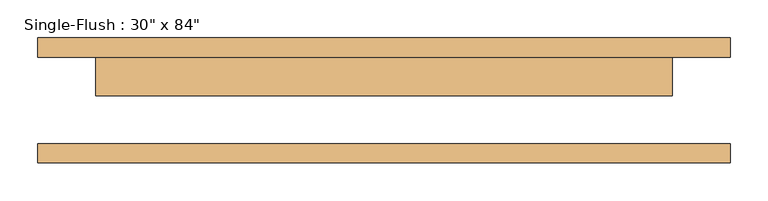
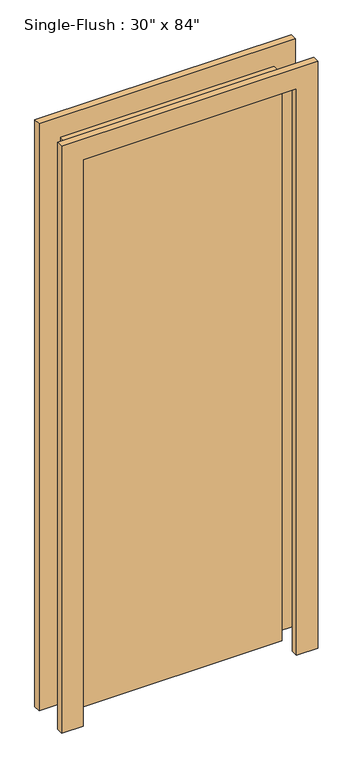
"""IFC4 building model written with IfcOpenShell, lengths in millimetres: door geometry."""

from ifc_helpers import new_model, si_unit, frame, origin, origin_with_axes, place, context, project, spatial, polyline, outline, extrude, source, transform, mapped, element, save


def door_214872d5(model_context):
    return source(origin(), model_context, "Body", "SweptSolid", [
        extrude(outline(polyline([(2209.8, -457.2), (0.0, -457.2), (0.0, -381.0), (2133.6, -381.0), (2133.6, 381.0), (0.0, 381.0), (0.0, 457.2), (2209.8, 457.2), (2209.8, -457.2)])), frame((0.0, 57.15, 0.0), z_axis=(0.0, 1.0, 0.0), x_axis=(0.0, 0.0, 1.0)), (0.0, 0.0, 1.0), 25.4),
        extrude(outline(polyline([(2209.8, 457.2), (2209.8, -457.2), (0.0, -457.2), (0.0, -381.0), (2133.6, -381.0), (2133.6, 381.0), (0.0, 381.0), (0.0, 457.2), (2209.8, 457.2)])), frame((0.0, -82.55, 0.0), z_axis=(0.0, 1.0, 0.0), x_axis=(0.0, 0.0, 1.0)), (0.0, 0.0, 1.0), 25.4),
        extrude(outline(polyline([(381.0, 6.35), (-381.0, 6.35), (-381.0, 57.15), (381.0, 57.15), (381.0, 6.35)])), origin_with_axes(), (0.0, 0.0, 1.0), 2133.6),
    ])


if __name__ == "__main__":
    model = new_model("IFC4")
    model_context = context("Model", 3, world=origin())
    ifc_project = project(units=[si_unit("LENGTHUNIT", "METRE", prefix="MILLI")], contexts=[model_context])
    site = spatial("IfcSite", under=ifc_project)
    building = spatial("IfcBuilding", under=site)
    placement = place(None, origin())
    door_shape = door_214872d5(model_context)
    element("IfcDoor", 1, ObjectType="Single-Flush : 30\" x 84\"", at=placement, inside=building, context=model_context, shape_type="MappedRepresentation", body=[
        mapped(door_shape, transform((0.0, 0.0, 0.0), x_axis=(1.0, 0.0, 0.0), y_axis=(0.0, 1.0, 0.0), z_axis=(0.0, 0.0, 1.0))),
    ])
    save(model, "model.ifc")

# Revit data of these elements
# Type "Single-Flush : 30\" x 84\""
#   Type Mark = "4"
#   Construction Type Id = "MDOOR"
#   Assembly Code = "C1020"
#   Analytic Construction = "Metal"
#   Thickness = 0' - 2"
#   Heat Transfer Coefficient (U) = 0.651978 BTU/(h·ft²·°F)
#   Height = 7' - 0"
#   Trim Projection Ext = 0' - 1"
#   Trim Projection Int = 0' - 1"
#   Trim Width = 0' - 3"
#   Width = 2' - 6"
#   Define Thermal Properties by = 1
#   Define Thermal Properties by = 1
#   Door Material = Door - Panel
#   Frame Material = Door - Frame
#   Visual Light Transmittance = 0
#   Solar Heat Gain Coefficient = 0
#   Function = (empty or 0)
#   Wall Closure = (empty or 0)
# Element 1 (IfcDoor, "Single-Flush : 30\" x 84\"")
#   Materials on its faces: "Door - Frame", "Door - Panel"
# Materials
#   "Door - Panel": class "Wood", colour RGB 210 159 95, transparency 0, Cost = 0
#   "Door - Frame": colour RGB 118 70 51, transparency 0, Cost = 0
